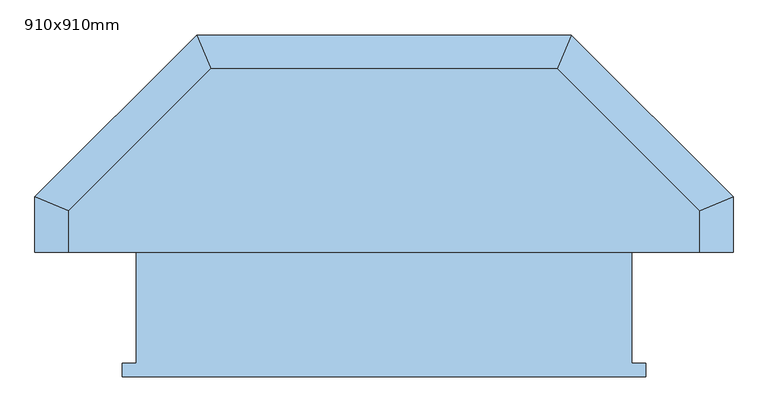
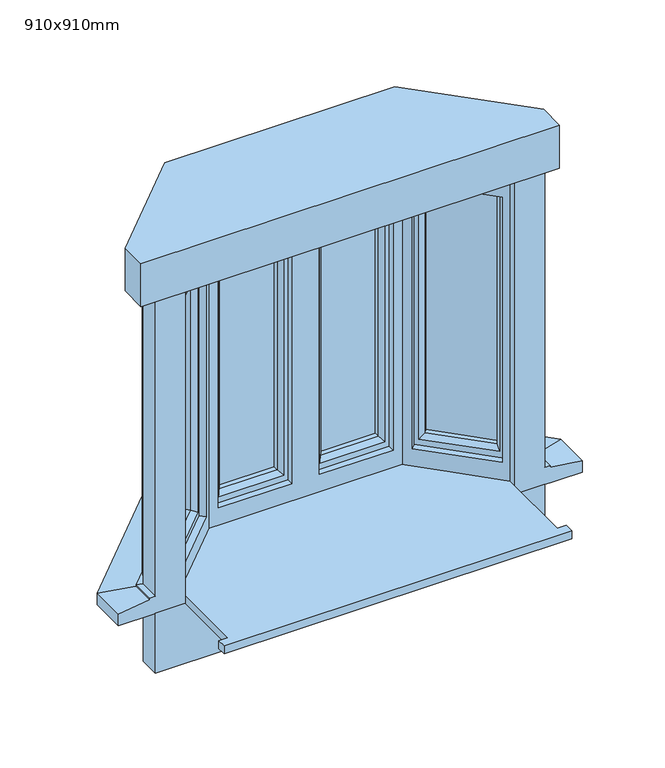
"""IFC4 building model written with IfcOpenShell, lengths in millimetres: window geometry, 910x910mm."""

from ifc_helpers import new_model, si_unit, frame, origin, place, context, project, spatial, polyline, outline, extrude, faceted_brep, source, transform, mapped, element, save


def window_910x910mm_67ef725a(model_context):
    return source(origin(), model_context, "Body", "SolidModel", [
        extrude(outline(polyline([(-1148.0, 186.004836), (-887.4810921, 446.5237439), (-252.5189079, 446.5237439), (8.0, 186.004836), (8.0, 110.0565678), (-1148.0, 110.0565678), (-1148.0, 186.004836)])), frame((0.0, 0.0, 2110.0), z_axis=(0.0, 0.0, 1.0), x_axis=(1.0, 0.0, 0.0)), (0.0, 0.0, 1.0), 125.0),
        extrude(outline(polyline([(-32.0, 169.4362935), (-32.0, 110.0565678), (-1108.0, 110.0565678), (-1108.0, 169.4362935), (-870.9125497, 406.5237439), (-269.0874503, 406.5237439), (-32.0, 169.4362935)])), frame((0.0, 0.0, 1025.0), z_axis=(0.0, 0.0, 1.0), x_axis=(1.0, 0.0, 0.0)), (0.0, 0.0, 1.0), 175.0),
        extrude(outline(polyline([(-90.0, -118.1434322), (-1050.0, -118.1434322), (-1050.0, -93.1434322), (-1025.0, -93.1434322), (-1025.0, 135.0565678), (-836.532824, 323.5237439), (-303.467176, 323.5237439), (-115.0, 135.0565678), (-115.0, -93.1434322), (-90.0, -93.1434322), (-90.0, -118.1434322)])), frame((0.0, 0.0, 1200.0), z_axis=(0.0, 0.0, 1.0), x_axis=(1.0, 0.0, 0.0)), (0.0, 0.0, 1.0), 24.0),
        faceted_brep([(-1025.0, 110.0565678, 1200.0), (-1025.0, 135.0565678, 1200.0), (-1025.0, 135.0565678, 2110.0), (-1025.0, 110.0565678, 2110.0), (-1108.0, 110.0565678, 1251.0), (-1123.0, 110.0565678, 1249.68767), (-1123.0, 110.0565678, 1244.7449676), (-1210.5, 110.0565678, 1233.8088847), (-1210.5, 110.0565678, 1200.0), (-1108.0, 110.0565678, 2110.0), (-1108.0, 169.4362935, 1251.0), (-1108.0, 169.4362935, 2110.0), (-870.9125497, 406.5237439, 2110.0), (-870.9125497, 406.5237439, 1251.0), (-1083.6898628, 193.7464307, 2070.0), (-1083.6898628, 193.7464307, 1263.0), (-900.1724343, 377.2638592, 1263.0), (-900.1724343, 377.2638592, 2070.0), (-1037.7279221, 147.7844899, 2070.0), (-1037.7279221, 147.7844899, 1263.0), (-854.2104935, 331.3019184, 1263.0), (-854.2104935, 331.3019184, 2070.0), (-1025.0, 160.5124119, 1275.0), (-866.9384156, 318.5739964, 1275.0), (-866.9384156, 318.5739964, 2050.0), (-1025.0, 160.5124119, 2050.0), (-1012.2720779, 147.7844899, 1275.0), (-1012.2720779, 147.7844899, 2050.0), (-836.532824, 323.5237439, 1200.0), (-836.532824, 323.5237439, 2110.0), (-854.2104935, 305.8460743, 2050.0), (-854.2104935, 305.8460743, 1275.0), (-269.0874503, 406.5237439, 2110.0), (-269.0874503, 406.5237439, 1251.0), (-310.467176, 406.5237439, 1263.0), (-310.467176, 406.5237439, 2070.0), (-550.0, 406.5237439, 2070.0), (-550.0, 406.5237439, 1263.0), (-829.532824, 406.5237439, 2070.0), (-829.532824, 406.5237439, 1263.0), (-590.0, 406.5237439, 1263.0), (-590.0, 406.5237439, 2070.0), (-829.532824, 341.5237439, 2070.0), (-829.532824, 341.5237439, 1263.0), (-310.467176, 341.5237439, 1263.0), (-550.0, 341.5237439, 1263.0), (-550.0, 341.5237439, 2070.0), (-310.467176, 341.5237439, 2070.0), (-532.0, 341.5237439, 1275.0), (-328.467176, 341.5237439, 1275.0), (-328.467176, 341.5237439, 2050.0), (-532.0, 341.5237439, 2050.0), (-590.0, 341.5237439, 1263.0), (-590.0, 341.5237439, 2070.0), (-811.532824, 341.5237439, 1275.0), (-608.0, 341.5237439, 1275.0), (-608.0, 341.5237439, 2050.0), (-811.532824, 341.5237439, 2050.0), (-811.532824, 323.5237439, 1275.0), (-811.532824, 323.5237439, 2050.0), (-303.467176, 323.5237439, 1200.0), (-303.467176, 323.5237439, 2110.0), (-608.0, 323.5237439, 2050.0), (-608.0, 323.5237439, 1275.0), (-532.0, 323.5237439, 1275.0), (-532.0, 323.5237439, 2050.0), (-328.467176, 323.5237439, 2050.0), (-328.467176, 323.5237439, 1275.0), (-115.0, 135.0565678, 1200.0), (-115.0, 135.0565678, 2110.0), (-285.7895065, 305.8460743, 1275.0), (-285.7895065, 305.8460743, 2050.0), (-127.7279221, 147.7844899, 2050.0), (-127.7279221, 147.7844899, 1275.0), (-32.0, 169.4362935, 2110.0), (-32.0, 169.4362935, 1251.0), (-239.8275657, 377.2638592, 2070.0), (-239.8275657, 377.2638592, 1263.0), (-56.3101372, 193.7464307, 1263.0), (-56.3101372, 193.7464307, 2070.0), (-285.7895065, 331.3019184, 2070.0), (-285.7895065, 331.3019184, 1263.0), (-102.2720779, 147.7844899, 1263.0), (-102.2720779, 147.7844899, 2070.0), (-273.0615844, 318.5739964, 1275.0), (-115.0, 160.5124119, 1275.0), (-115.0, 160.5124119, 2050.0), (-273.0615844, 318.5739964, 2050.0), (-32.0, 110.0565678, 1251.0), (-32.0, 110.0565678, 2110.0), (-115.0, 110.0565678, 1200.0), (70.5, 110.0565678, 1200.0), (70.5, 110.0565678, 1233.8088847), (-17.0, 110.0565678, 1244.7449676), (-17.0, 110.0565678, 1249.68767), (-115.0, 110.0565678, 2110.0), (-1123.0, 175.6494969, 1249.68767), (-1123.0, 175.6494969, 1244.7449676), (-1210.5, 211.8931836, 1233.8088847), (-1210.5, 211.8931836, 1200.0), (-913.3694398, 509.0237439, 1200.0), (-226.6305602, 509.0237439, 1200.0), (70.5, 211.8931836, 1200.0), (-877.1257531, 421.5237439, 1249.68767), (-877.1257531, 421.5237439, 1244.7449676), (-913.3694398, 509.0237439, 1233.8088847), (-262.8742469, 421.5237439, 1249.68767), (-262.8742469, 421.5237439, 1244.7449676), (-226.6305602, 509.0237439, 1233.8088847), (-17.0, 175.6494969, 1249.68767), (-17.0, 175.6494969, 1244.7449676), (70.5, 211.8931836, 1233.8088847)], [[[0, 1, 2, 3]], [[4, 5, 6, 7, 8, 0, 3, 9]], [[10, 4, 9, 11]], [[10, 11, 12, 13], [14, 15, 16, 17]], [[15, 14, 18, 19]], [[20, 19, 18, 21], [22, 23, 24, 25]], [[26, 22, 25, 27]], [[2, 1, 28, 29], [26, 27, 30, 31]], [[23, 31, 30, 24]], [[17, 16, 20, 21]], [[13, 12, 32, 33], [34, 35, 36, 37], [38, 39, 40, 41]], [[39, 38, 42, 43]], [[44, 45, 46, 47], [48, 49, 50, 51]], [[52, 43, 42, 53], [54, 55, 56, 57]], [[58, 54, 57, 59]], [[29, 28, 60, 61], [58, 59, 62, 63], [64, 65, 66, 67]], [[61, 60, 68, 69], [70, 71, 72, 73]], [[49, 67, 66, 50]], [[35, 34, 44, 47]], [[33, 32, 74, 75], [76, 77, 78, 79]], [[77, 76, 80, 81]], [[82, 81, 80, 83], [84, 85, 86, 87]], [[70, 84, 87, 71]], [[85, 73, 72, 86]], [[79, 78, 82, 83]], [[88, 75, 74, 89]], [[90, 91, 92, 93, 94, 88, 89, 95]], [[69, 68, 90, 95]], [[41, 40, 52, 53]], [[37, 36, 46, 45]], [[64, 48, 51, 65]], [[55, 63, 62, 56]], [[26, 31, 23, 22]], [[49, 48, 64, 67]], [[55, 54, 58, 63]], [[70, 73, 85, 84]], [[16, 15, 19, 20]], [[34, 37, 45, 44]], [[40, 39, 43, 52]], [[78, 77, 81, 82]], [[5, 4, 10, 96]], [[6, 5, 96, 97]], [[7, 6, 97, 98]], [[8, 7, 98, 99]], [[0, 8, 99, 100, 101, 102, 91, 90, 68, 60, 28, 1]], [[96, 10, 13, 103]], [[97, 96, 103, 104]], [[98, 97, 104, 105]], [[99, 98, 105, 100]], [[103, 13, 33, 106]], [[104, 103, 106, 107]], [[105, 104, 107, 108]], [[101, 100, 105, 108]], [[106, 33, 75, 109]], [[107, 106, 109, 110]], [[108, 107, 110, 111]], [[102, 101, 108, 111]], [[109, 75, 88, 94]], [[110, 109, 94, 93]], [[111, 110, 93, 92]], [[91, 102, 111, 92]], [[9, 3, 2, 29, 61, 69, 95, 89, 74, 32, 12, 11]], [[14, 17, 21, 18]], [[47, 46, 36, 35]], [[53, 42, 38, 41]], [[76, 79, 83, 80]], [[25, 24, 30, 27]], [[57, 56, 62, 59]], [[66, 65, 51, 50]], [[87, 86, 72, 71]]]),
        faceted_brep([(-1090.7609307, 186.6753629, 2080.0), (-1094.8434136, 190.7578458, 2080.0), (-1094.8434136, 190.7578458, 1253.0), (-1090.7609307, 186.6753629, 1253.0), (-1037.7279221, 147.7844899, 2070.0), (-1083.6898628, 193.7464307, 2070.0), (-1083.6898628, 193.7464307, 1263.0), (-1037.7279221, 147.7844899, 1263.0), (-1019.6916786, 186.3167889, 2030.0), (-1016.6193971, 168.8930148, 2040.1480377), (-1016.6193971, 168.8930148, 1292.8519623), (-1019.6916786, 186.3167889, 1303.0), (-1029.9497475, 196.5748578, 2030.0), (-1029.9497475, 196.5748578, 1303.0), (-1053.991378, 206.4743527, 2040.0), (-1037.0208153, 189.50379, 2040.0), (-1037.0208153, 189.50379, 1293.0), (-1053.991378, 206.4743527, 1293.0), (-1059.4880745, 226.1131848, 2030.0), (-1046.9203102, 213.5454205, 2030.0), (-1046.9203102, 213.5454205, 1303.0), (-1059.4880745, 226.1131848, 1303.0), (-1075.9065689, 217.8596562, 2047.4457548), (-1075.9065689, 217.8596562, 1285.5542452), (-1091.3000258, 202.4661993, 2069.2153903), (-1091.3000258, 202.4661993, 1263.7846097), (-897.1838494, 388.4174099, 1253.0), (-893.1013665, 384.334927, 1253.0), (-900.1724343, 377.2638592, 1263.0), (-854.2104935, 331.3019184, 1263.0), (-875.3190185, 310.1933935, 1292.8519623), (-892.7427925, 313.265675, 1303.0), (-903.0008614, 323.5237439, 1303.0), (-895.9297936, 330.5948117, 1293.0), (-912.9003563, 347.5653744, 1293.0), (-919.9714242, 340.4943066, 1303.0), (-932.5391884, 353.0620709, 1303.0), (-924.2856598, 369.4805653, 1285.5542452), (-908.8922029, 384.8740222, 1263.7846097), (-897.1838494, 388.4174099, 2080.0), (-893.1013665, 384.334927, 2080.0), (-900.1724343, 377.2638592, 2070.0), (-854.2104935, 331.3019184, 2070.0), (-875.3190185, 310.1933935, 2040.1480377), (-892.7427925, 313.265675, 2030.0), (-903.0008614, 323.5237439, 2030.0), (-895.9297936, 330.5948117, 2040.0), (-912.9003563, 347.5653744, 2040.0), (-919.9714242, 340.4943066, 2030.0), (-932.5391884, 353.0620709, 2030.0), (-924.2856598, 369.4805653, 2047.4457548), (-908.8922029, 384.8740222, 2069.2153903)], [[[0, 1, 2, 3]], [[4, 5, 6, 7]], [[8, 9, 10, 11]], [[12, 8, 11, 13]], [[14, 15, 16, 17]], [[18, 19, 20, 21]], [[22, 18, 21, 23]], [[1, 24, 25, 2]], [[3, 2, 26, 27]], [[7, 6, 28, 29]], [[11, 10, 30, 31]], [[13, 11, 31, 32]], [[17, 16, 33, 34]], [[21, 20, 35, 36]], [[23, 21, 36, 37]], [[2, 25, 38, 26]], [[27, 26, 39, 40]], [[29, 28, 41, 42]], [[31, 30, 43, 44]], [[32, 31, 44, 45]], [[34, 33, 46, 47]], [[36, 35, 48, 49]], [[37, 36, 49, 50]], [[26, 38, 51, 39]], [[40, 39, 1, 0]], [[3, 27, 40, 0], [5, 41, 28, 6]], [[42, 41, 5, 4]], [[7, 29, 42, 4], [9, 43, 30, 10]], [[44, 43, 9, 8]], [[45, 44, 8, 12]], [[15, 46, 33, 16], [13, 32, 45, 12]], [[47, 46, 15, 14]], [[17, 34, 47, 14], [19, 48, 35, 20]], [[49, 48, 19, 18]], [[50, 49, 18, 22]], [[24, 51, 38, 25], [23, 37, 50, 22]], [[39, 51, 24, 1]]]),
        faceted_brep([(-839.532824, 406.5237439, 2080.0), (-839.532824, 412.2972465, 2080.0), (-839.532824, 412.2972465, 1253.0), (-839.532824, 406.5237439, 1253.0), (-829.532824, 341.5237439, 2070.0), (-829.532824, 406.5237439, 2070.0), (-829.532824, 406.5237439, 1263.0), (-829.532824, 341.5237439, 1263.0), (-789.532824, 356.0166437, 2030.0), (-799.6808617, 341.5237439, 2040.1480377), (-799.6808617, 341.5237439, 1292.8519623), (-789.532824, 356.0166437, 1303.0), (-789.532824, 370.5237439, 2030.0), (-789.532824, 370.5237439, 1303.0), (-799.532824, 394.5237439, 2040.0), (-799.532824, 370.5237439, 2040.0), (-799.532824, 370.5237439, 1293.0), (-799.532824, 394.5237439, 1293.0), (-789.532824, 412.2972465, 2030.0), (-789.532824, 394.5237439, 2030.0), (-789.532824, 394.5237439, 1303.0), (-789.532824, 412.2972465, 1303.0), (-806.9785788, 418.0707492, 2047.4457548), (-806.9785788, 418.0707492, 1285.5542452), (-828.7482143, 418.0707492, 2069.2153903), (-828.7482143, 418.0707492, 1263.7846097), (-580.0, 412.2972465, 1253.0), (-580.0, 406.5237439, 1253.0), (-590.0, 406.5237439, 1263.0), (-590.0, 341.5237439, 1263.0), (-619.8519623, 341.5237439, 1292.8519623), (-630.0, 356.0166437, 1303.0), (-630.0, 370.5237439, 1303.0), (-620.0, 370.5237439, 1293.0), (-620.0, 394.5237439, 1293.0), (-630.0, 394.5237439, 1303.0), (-630.0, 412.2972465, 1303.0), (-612.5542452, 418.0707492, 1285.5542452), (-590.7846097, 418.0707492, 1263.7846097), (-580.0, 412.2972465, 2080.0), (-580.0, 406.5237439, 2080.0), (-590.0, 406.5237439, 2070.0), (-590.0, 341.5237439, 2070.0), (-619.8519623, 341.5237439, 2040.1480377), (-630.0, 356.0166437, 2030.0), (-630.0, 370.5237439, 2030.0), (-620.0, 370.5237439, 2040.0), (-620.0, 394.5237439, 2040.0), (-630.0, 394.5237439, 2030.0), (-630.0, 412.2972465, 2030.0), (-612.5542452, 418.0707492, 2047.4457548), (-590.7846097, 418.0707492, 2069.2153903)], [[[0, 1, 2, 3]], [[4, 5, 6, 7]], [[8, 9, 10, 11]], [[12, 8, 11, 13]], [[14, 15, 16, 17]], [[18, 19, 20, 21]], [[22, 18, 21, 23]], [[1, 24, 25, 2]], [[3, 2, 26, 27]], [[7, 6, 28, 29]], [[11, 10, 30, 31]], [[13, 11, 31, 32]], [[17, 16, 33, 34]], [[21, 20, 35, 36]], [[23, 21, 36, 37]], [[2, 25, 38, 26]], [[27, 26, 39, 40]], [[29, 28, 41, 42]], [[31, 30, 43, 44]], [[32, 31, 44, 45]], [[34, 33, 46, 47]], [[36, 35, 48, 49]], [[37, 36, 49, 50]], [[26, 38, 51, 39]], [[40, 39, 1, 0]], [[3, 27, 40, 0], [5, 41, 28, 6]], [[42, 41, 5, 4]], [[7, 29, 42, 4], [9, 43, 30, 10]], [[44, 43, 9, 8]], [[45, 44, 8, 12]], [[15, 46, 33, 16], [13, 32, 45, 12]], [[47, 46, 15, 14]], [[17, 34, 47, 14], [19, 48, 35, 20]], [[49, 48, 19, 18]], [[50, 49, 18, 22]], [[24, 51, 38, 25], [23, 37, 50, 22]], [[39, 51, 24, 1]]]),
        faceted_brep([(-560.0, 406.5237439, 2080.0), (-560.0, 412.2972465, 2080.0), (-560.0, 412.2972465, 1253.0), (-560.0, 406.5237439, 1253.0), (-550.0, 341.5237439, 2070.0), (-550.0, 406.5237439, 2070.0), (-550.0, 406.5237439, 1263.0), (-550.0, 341.5237439, 1263.0), (-510.0, 356.0166437, 2030.0), (-520.1480377, 341.5237439, 2040.1480377), (-520.1480377, 341.5237439, 1292.8519623), (-510.0, 356.0166437, 1303.0), (-510.0, 370.5237439, 2030.0), (-510.0, 370.5237439, 1303.0), (-520.0, 394.5237439, 2040.0), (-520.0, 370.5237439, 2040.0), (-520.0, 370.5237439, 1293.0), (-520.0, 394.5237439, 1293.0), (-510.0, 412.2972465, 2030.0), (-510.0, 394.5237439, 2030.0), (-510.0, 394.5237439, 1303.0), (-510.0, 412.2972465, 1303.0), (-527.4457548, 418.0707492, 2047.4457548), (-527.4457548, 418.0707492, 1285.5542452), (-549.2153903, 418.0707492, 2069.2153903), (-549.2153903, 418.0707492, 1263.7846097), (-300.467176, 412.2972465, 1253.0), (-300.467176, 406.5237439, 1253.0), (-310.467176, 406.5237439, 1263.0), (-310.467176, 341.5237439, 1263.0), (-340.3191383, 341.5237439, 1292.8519623), (-350.467176, 356.0166437, 1303.0), (-350.467176, 370.5237439, 1303.0), (-340.467176, 370.5237439, 1293.0), (-340.467176, 394.5237439, 1293.0), (-350.467176, 394.5237439, 1303.0), (-350.467176, 412.2972465, 1303.0), (-333.0214212, 418.0707492, 1285.5542452), (-311.2517857, 418.0707492, 1263.7846097), (-300.467176, 412.2972465, 2080.0), (-300.467176, 406.5237439, 2080.0), (-310.467176, 406.5237439, 2070.0), (-310.467176, 341.5237439, 2070.0), (-340.3191383, 341.5237439, 2040.1480377), (-350.467176, 356.0166437, 2030.0), (-350.467176, 370.5237439, 2030.0), (-340.467176, 370.5237439, 2040.0), (-340.467176, 394.5237439, 2040.0), (-350.467176, 394.5237439, 2030.0), (-350.467176, 412.2972465, 2030.0), (-333.0214212, 418.0707492, 2047.4457548), (-311.2517857, 418.0707492, 2069.2153903)], [[[0, 1, 2, 3]], [[4, 5, 6, 7]], [[8, 9, 10, 11]], [[12, 8, 11, 13]], [[14, 15, 16, 17]], [[18, 19, 20, 21]], [[22, 18, 21, 23]], [[1, 24, 25, 2]], [[3, 2, 26, 27]], [[7, 6, 28, 29]], [[11, 10, 30, 31]], [[13, 11, 31, 32]], [[17, 16, 33, 34]], [[21, 20, 35, 36]], [[23, 21, 36, 37]], [[2, 25, 38, 26]], [[27, 26, 39, 40]], [[29, 28, 41, 42]], [[31, 30, 43, 44]], [[32, 31, 44, 45]], [[34, 33, 46, 47]], [[36, 35, 48, 49]], [[37, 36, 49, 50]], [[26, 38, 51, 39]], [[40, 39, 1, 0]], [[3, 27, 40, 0], [5, 41, 28, 6]], [[42, 41, 5, 4]], [[7, 29, 42, 4], [9, 43, 30, 10]], [[44, 43, 9, 8]], [[45, 44, 8, 12]], [[15, 46, 33, 16], [13, 32, 45, 12]], [[47, 46, 15, 14]], [[17, 34, 47, 14], [19, 48, 35, 20]], [[49, 48, 19, 18]], [[50, 49, 18, 22]], [[24, 51, 38, 25], [23, 37, 50, 22]], [[39, 51, 24, 1]]]),
        faceted_brep([(-246.8986335, 384.334927, 2080.0), (-242.8161506, 388.4174099, 2080.0), (-242.8161506, 388.4174099, 1253.0), (-246.8986335, 384.334927, 1253.0), (-285.7895065, 331.3019184, 2070.0), (-239.8275657, 377.2638592, 2070.0), (-239.8275657, 377.2638592, 1263.0), (-285.7895065, 331.3019184, 1263.0), (-247.2572075, 313.265675, 2030.0), (-264.6809815, 310.1933935, 2040.1480377), (-264.6809815, 310.1933935, 1292.8519623), (-247.2572075, 313.265675, 1303.0), (-236.9991386, 323.5237439, 2030.0), (-236.9991386, 323.5237439, 1303.0), (-227.0996437, 347.5653744, 2040.0), (-244.0702064, 330.5948117, 2040.0), (-244.0702064, 330.5948117, 1293.0), (-227.0996437, 347.5653744, 1293.0), (-207.4608116, 353.0620709, 2030.0), (-220.0285758, 340.4943066, 2030.0), (-220.0285758, 340.4943066, 1303.0), (-207.4608116, 353.0620709, 1303.0), (-215.7143402, 369.4805653, 2047.4457548), (-215.7143402, 369.4805653, 1285.5542452), (-231.1077971, 384.8740222, 2069.2153903), (-231.1077971, 384.8740222, 1263.7846097), (-45.1565864, 190.7578458, 1253.0), (-49.2390693, 186.6753629, 1253.0), (-56.3101372, 193.7464307, 1263.0), (-102.2720779, 147.7844899, 1263.0), (-123.3806029, 168.8930148, 1292.8519623), (-120.3083214, 186.3167889, 1303.0), (-110.0502525, 196.5748578, 1303.0), (-102.9791847, 189.50379, 1293.0), (-86.008622, 206.4743527, 1293.0), (-93.0796898, 213.5454205, 1303.0), (-80.5119255, 226.1131848, 1303.0), (-64.0934311, 217.8596562, 1285.5542452), (-48.6999742, 202.4661993, 1263.7846097), (-45.1565864, 190.7578458, 2080.0), (-49.2390693, 186.6753629, 2080.0), (-56.3101372, 193.7464307, 2070.0), (-102.2720779, 147.7844899, 2070.0), (-123.3806029, 168.8930148, 2040.1480377), (-120.3083214, 186.3167889, 2030.0), (-110.0502525, 196.5748578, 2030.0), (-102.9791847, 189.50379, 2040.0), (-86.008622, 206.4743527, 2040.0), (-93.0796898, 213.5454205, 2030.0), (-80.5119255, 226.1131848, 2030.0), (-64.0934311, 217.8596562, 2047.4457548), (-48.6999742, 202.4661993, 2069.2153903)], [[[0, 1, 2, 3]], [[4, 5, 6, 7]], [[8, 9, 10, 11]], [[12, 8, 11, 13]], [[14, 15, 16, 17]], [[18, 19, 20, 21]], [[22, 18, 21, 23]], [[1, 24, 25, 2]], [[3, 2, 26, 27]], [[7, 6, 28, 29]], [[11, 10, 30, 31]], [[13, 11, 31, 32]], [[17, 16, 33, 34]], [[21, 20, 35, 36]], [[23, 21, 36, 37]], [[2, 25, 38, 26]], [[27, 26, 39, 40]], [[29, 28, 41, 42]], [[31, 30, 43, 44]], [[32, 31, 44, 45]], [[34, 33, 46, 47]], [[36, 35, 48, 49]], [[37, 36, 49, 50]], [[26, 38, 51, 39]], [[40, 39, 1, 0]], [[3, 27, 40, 0], [5, 41, 28, 6]], [[42, 41, 5, 4]], [[7, 29, 42, 4], [9, 43, 30, 10]], [[44, 43, 9, 8]], [[45, 44, 8, 12]], [[15, 46, 33, 16], [13, 32, 45, 12]], [[47, 46, 15, 14]], [[17, 34, 47, 14], [19, 48, 35, 20]], [[49, 48, 19, 18]], [[50, 49, 18, 22]], [[24, 51, 38, 25], [23, 37, 50, 22]], [[39, 51, 24, 1]]]),
        extrude(outline(polyline([(-340.467176, 370.5237439), (-520.0, 370.5237439), (-520.0, 394.5237439), (-340.467176, 394.5237439), (-340.467176, 370.5237439)])), frame((0.0, 0.0, 1285.5542452), z_axis=(0.0, 0.0, 1.0), x_axis=(1.0, 0.0, 0.0)), (0.0, 0.0, 1.0), 761.8915096),
        extrude(outline(polyline([(-620.0, 370.5237439), (-799.532824, 370.5237439), (-799.532824, 394.5237439), (-620.0, 394.5237439), (-620.0, 370.5237439)])), frame((0.0, 0.0, 1285.5542452), z_axis=(0.0, 0.0, 1.0), x_axis=(1.0, 0.0, 0.0)), (0.0, 0.0, 1.0), 761.8915096),
        extrude(outline(polyline([(-1053.991378, 206.4743527), (-912.9003563, 347.5653744), (-895.9297936, 330.5948117), (-1037.0208153, 189.50379), (-1053.991378, 206.4743527)])), frame((0.0, 0.0, 1292.8519623), z_axis=(0.0, 0.0, 1.0), x_axis=(1.0, 0.0, 0.0)), (0.0, 0.0, 1.0), 747.2960754),
        extrude(outline(polyline([(-102.9791847, 189.50379), (-244.0702064, 330.5948117), (-227.0996437, 347.5653744), (-86.008622, 206.4743527), (-102.9791847, 189.50379)])), frame((0.0, 0.0, 1293.0), z_axis=(0.0, 0.0, 1.0), x_axis=(1.0, 0.0, 0.0)), (0.0, 0.0, 1.0), 747.0),
    ])


if __name__ == "__main__":
    model = new_model("IFC4")
    model_context = context("Model", 3, world=origin())
    ifc_project = project(units=[si_unit("LENGTHUNIT", "METRE", prefix="MILLI")], contexts=[model_context])
    site = spatial("IfcSite", under=ifc_project)
    building = spatial("IfcBuilding", under=site)
    placement = place(None, origin())
    window_910x910mm_shape = window_910x910mm_67ef725a(model_context)
    element("IfcWindow", 1, ObjectType="910x910mm", at=placement, inside=building, context=model_context, shape_type="MappedRepresentation", body=[
        mapped(window_910x910mm_shape, transform((0.0, 0.0, 0.0), x_axis=(1.0, 0.0, 0.0), y_axis=(0.0, 1.0, 0.0), z_axis=(0.0, 0.0, 1.0))),
    ])
    save(model, "model.ifc")

# Revit data of these elements
# Type "910x910mm"
#   Type Mark = "18"
#   Operation = "UserDefined"
#   Construction Type Id = "GSP4R"
#   Keynote = "L10"
#   Analytic Construction = "1/8 in Pilkington single glazing"
#   Wrap Layers (Ext) from Ext = 0' - 4.03543"
#   Wrap Layers (Int) from Ext = 0' - 6.98819"
#   Window Board Projection = 0' - 0.98425"
#   Window Board Extention = 0' - 0.98425"
#   Visual Light Transmittance = 0.9
#   Solar Heat Gain Coefficient = 0.78
#   Heat Transfer Coefficient (U) = 0.6496 BTU/(h·ft²·°F)
#   Glazing Thickness = 0' - 0.94488"
#   DONT CHANGE - Splay Width = 0' - 7.41997"
#   Rough Width = 2' - 11.82677"
#   Rough Height = 2' - 11.82677"
#   Roof Thickness = 0' - 4.92126"
#   Roof Overhang = 0' - 1.5748"
#   Plinth Thickness = 0' - 6.88976"
#   Height = 2' - 11.82677"
#   Width = 2' - 11.82677"
#   Frame Depth = 0' - 2.55906"
#   Default Head Height = 6' - 11.07087"
#   Cill Depth = 0' - 3.44488"
#   Cavity Closer Width = 0' - 1.9685"
#   Cavity Closer Offset from Ext = 0' - 4.03543"
#   Cavity Closer Depth = 0' - 3.34646"
#   Vis - Cavity Closers = yes
#   Define Thermal Properties by = 1
#   Material Trim = Window Frame
#   Material Glass = Glass
#   Material Frame = Window Frame
#   Manufacturer = ""
#   Wall Closure = (empty or 0)
# Element 1 (IfcWindow, "910x910mm")
#   Materials on its faces: "Window Frame", "Glass"
# Materials
#   "Window Frame": colour RGB 249 249 249, transparency 0
#   "Glass": class "Glass", colour RGB 0 128 192, transparency 0.75, Description = "Soda Lime Glass", Cost = 0
